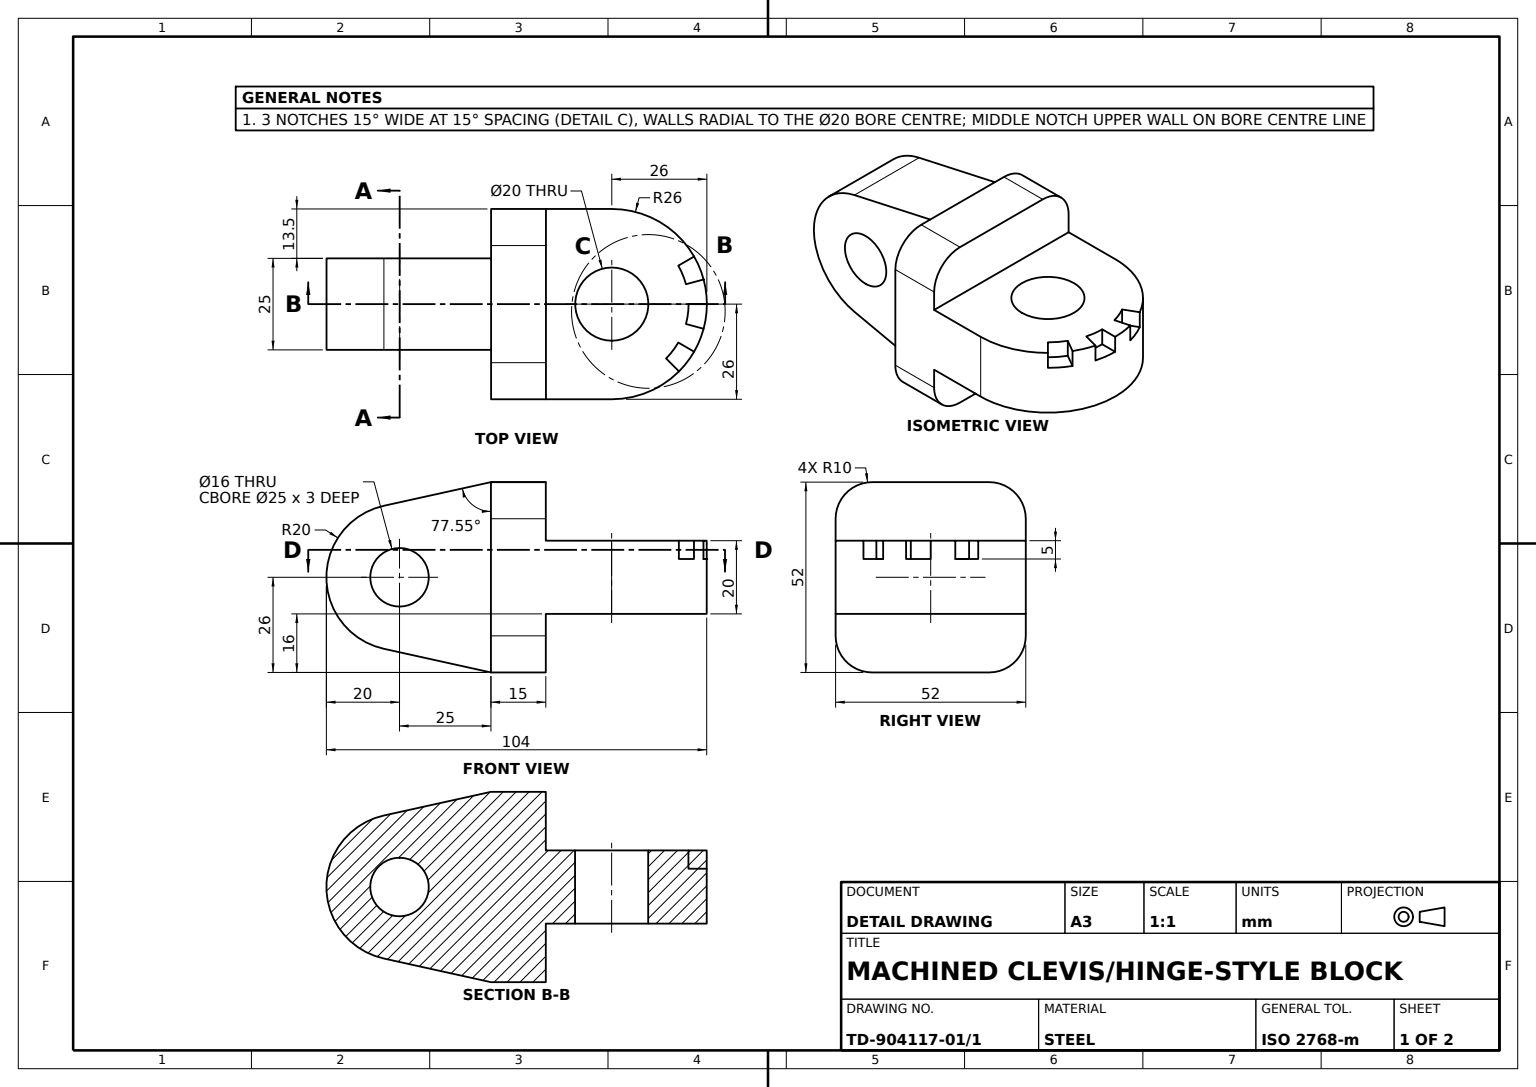
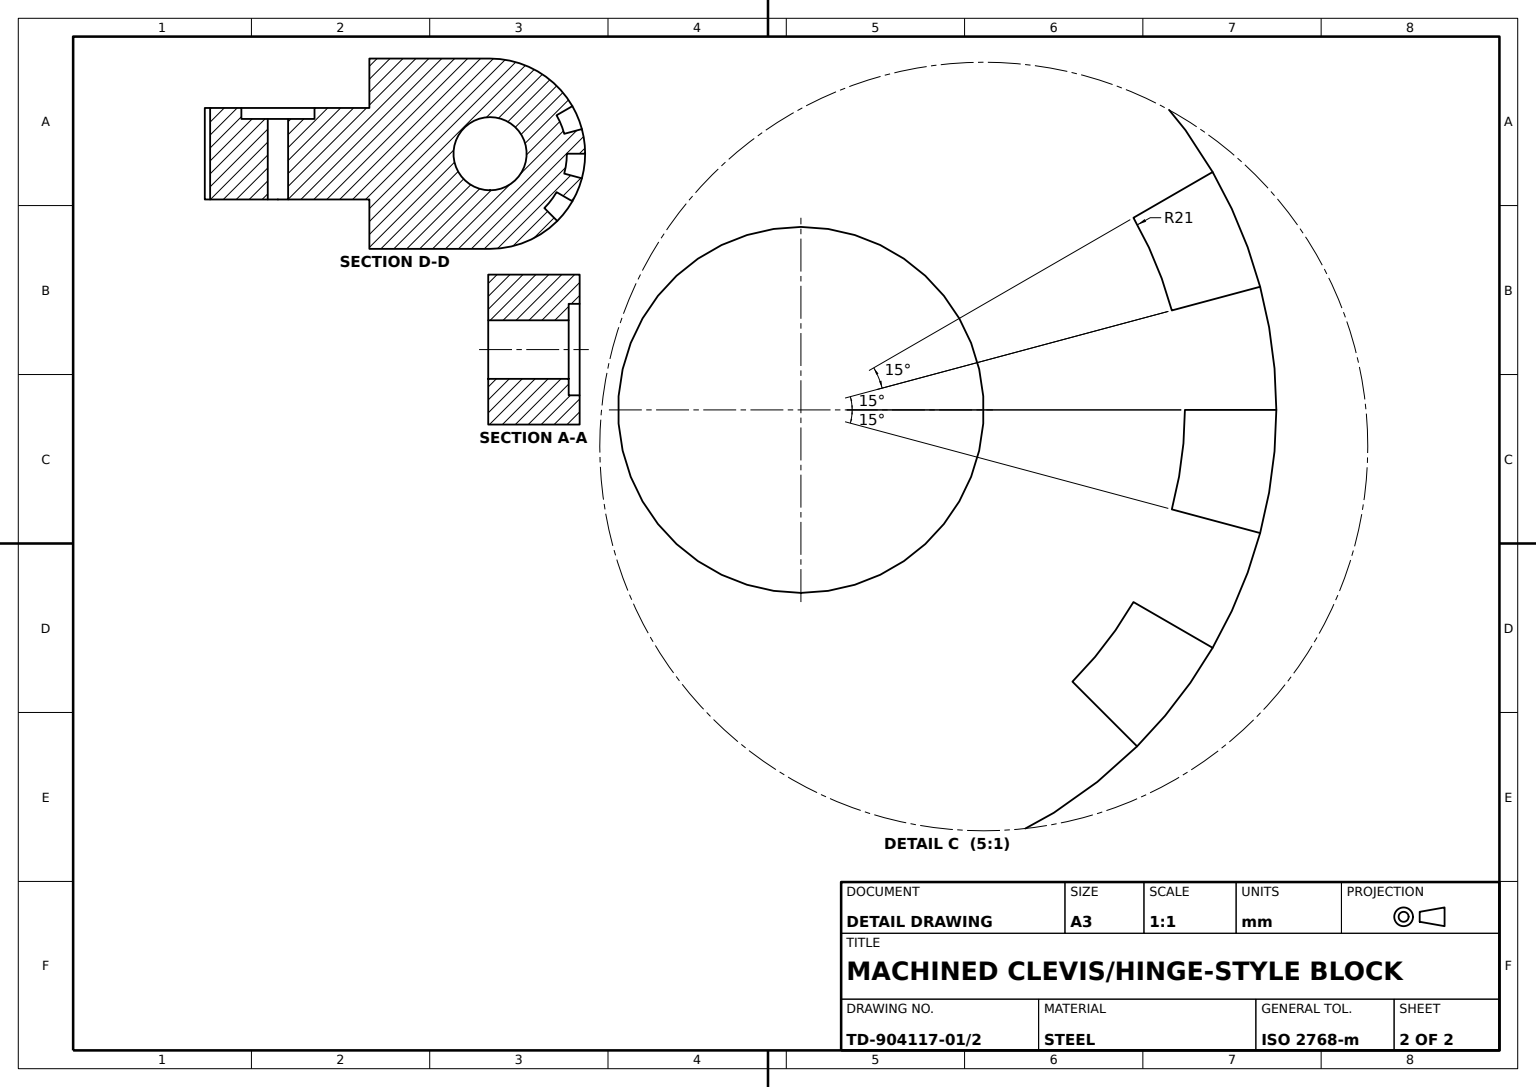
SolidWorks part; units mm, degrees
material "Plain Carbon Steel"
ref_plane "Front Plane" through (0, 0, 0) normal (0, 0, 1) x (1, 0, 0)
ref_plane "Top Plane" through (0, 0, 0) normal (0, 1, 0) x (1, 0, 0)
ref_plane "Right Plane" through (0, 0, 0) normal (1, 0, 0) x (0, 0, -1)
sketch "Base Block Profile Sketch" plane through (0, 0, 0) normal (0, 0, 1) x (1, 0, 0)
  line L0 (-16, 0) -> (16, 0)
  line L1 (26, 10) -> (26, 42)
  line L2 (16, 52) -> (-16, 52)
  line L3 (-26, 42) -> (-26, 10)
  arc A0 (-16, 0) -> (-26, 10) centre (-16, 10) cw
  arc A1 (16, 0) -> (26, 10) centre (16, 10) ccw
  arc A2 (26, 42) -> (16, 52) centre (16, 42) ccw
  arc A3 (-16, 52) -> (-26, 42) centre (-16, 42) ccw
  point P4 (0, 0)
  point P11 (26, 0)
  point P14 (26, 52)
  point P17 (-26, 52)
  dimension "D3" = 10
  dimension "D1" = 52
  dimension "D2" = 52
extrude "Rounded Base Block" add sketch "Base Block Profile Sketch" along normal blind 15
sketch "Upper Block Profile Sketch" plane through (-26, 0, 0) normal (-1, 0, 0) x (0, 0, 1)
  line L0 (15, 52) -> (15, 0)
  line L2 (15, 52) -> (44.311, 45.5298)
  line L3 (15, 0) -> (44.311, 6.4702)
  arc A0 (44.311, 6.4702) -> (44.311, 45.5298) centre (40, 26) ccw
  dimension "D2" = 20
  dimension "D1" = 25
  dimension "D3" = 19.5298
extrude "Upper Block" add sketch "Upper Block Profile Sketch" against normal blind 52
sketch "Upper Block Notch A Sketch" plane through (-26, 0, 0) normal (-1, 0, 0) x (0, 0, 1)
  line L0 (15, 52) -> (44.311, 45.5298)
  line L1 (15, 0) -> (44.311, 6.4702)
  line L2 (15, 52) -> (15, 0)
  arc A0 (44.311, 6.4702) -> (44.311, 45.5298) centre (40, 26) ccw
extrude "Upper Block Notch A" cut sketch "Upper Block Notch A Sketch" against normal blind 13.5
sketch "Upper Block Notch B Sketch" plane through (26, 0, 0) normal (1, 0, 0) x (0, 0, -1)
  line L0 (-15, 52) -> (-15, 0)
  line L1 (-15, 0) -> (-44.311, 6.4702)
  line L2 (-15, 52) -> (-44.311, 45.5298)
  arc A0 (-44.311, 45.5298) -> (-44.311, 6.4702) centre (-40, 26) ccw
extrude "Upper Block Notch B" cut sketch "Upper Block Notch B Sketch" against normal blind 13.5
sketch "Cross Block Profile Sketch" plane through (0, 52, 0) normal (0, 1, 0) x (1, 0, 0)
  line L1 (-26, 0) -> (-26, 18)
  line L2 (26, 0) -> (26, 18)
  line L3 (-26, 0) -> (26, 0)
  arc A0 (26, 18) -> (-26, 18) centre (0, 18) ccw
  dimension "D2" = 26
  dimension "D1" = 18
  dimension "D3" = 33
  dimension "D4" = 38.5
  dimension "D5" = 18
extrude "Cross Block" add sketch "Cross Block Profile Sketch" against normal blind 52
sketch "Cross Block Notch A Sketch" plane through (0, 52, 0) normal (0, 1, 0) x (1, 0, 0)
  line L0 (-26, 0) -> (26, 0)
  line L1 (26, 0) -> (26, 18)
  line L2 (-26, 0) -> (-26, 18)
  arc A0 (26, 18) -> (-26, 18) centre (0, 18) ccw
extrude "Cross Block Notch A" cut sketch "Cross Block Notch A Sketch" against normal blind 16
sketch "Cross Block Notch B Sketch" plane through (0, 0, 0) normal (0, -1, 0) x (1, 0, 0)
  line L0 (-26, 0) -> (26, 0)
  line L1 (26, 0) -> (26, -18)
  line L2 (-26, 0) -> (-26, -18)
  arc A0 (-26, -18) -> (26, -18) centre (0, -18) ccw
extrude "Cross Block Notch B" cut sketch "Cross Block Notch B Sketch" against normal blind 16
sketch "Bore Notch Teeth Sketch" plane through (0, 36, 0) normal (0, 1, 0) x (1, 0, 0)
  line L0 (0, 0) -> (0, 44)
  line L2 (-5.4352, 38.2844) -> (-6.7293, 43.1141)
  line L3 (5.4352, 38.2844) -> (6.7293, 43.1141)
  line L5 (-10.5, 36.1865) -> (-13, 40.5167)
  line L6 (14.8492, 32.8492) -> (18.3848, 36.3848)
  line L7 (10.5, 36.1865) -> (13, 40.5167)
  arc A0 (26, 18) -> (-26, 18) centre (0, 18) ccw construction
  arc A3 (14.8492, 32.8492) -> (10.5, 36.1865) centre (0, 18) ccw
  arc A4 (-5.4352, 38.2844) -> (-10.5, 36.1865) centre (0, 18) ccw
  arc A5 (18.3848, 36.3848) -> (13, 40.5167) centre (0, 18) ccw
  arc A6 (-6.7293, 43.1141) -> (-13, 40.5167) centre (0, 18) ccw
  arc A7 (5.4352, 38.2844) -> (0, 39) centre (0, 18) ccw
  arc A8 (6.7293, 43.1141) -> (0, 44) centre (0, 18) ccw
  arc M12 (26, 18) -> (-26, 18) centre (0, 18) ccw
  dimension "D1" = 15
  dimension "D3" = 15
  dimension "D7" = 21
  dimension "D2" = 15
  dimension "D4" = 15
  dimension "D5" = 75
  dimension "D6" = 4.3301
  dimension "D8" = 7.5648
  dimension "D9" = 13.0882
  dimension "D10" = 5
  dimension "D11" = 3.5355
extrude "Bore Notch Teeth Cut" cut sketch "Bore Notch Teeth Sketch" against normal blind 5 contours A4 L2 L5 M12 | A7 L3 L0 M12 | A3 L6 L7 M12
sketch "Cross Bore Ø10 Sketch" plane through (0, 36, 0) normal (0, 1, 0) x (1, 0, 0)
  circle A0 centre (0, 18) radius 10
  dimension "D1" = 10
extrude "Cross Bore Ø10" cut sketch "Cross Bore Ø10 Sketch" against normal blind 50
sketch "Counterbore Ø25 Sketch" plane through (-12.5, 0, 0) normal (-1, 0, 0) x (0, 0, 1)
  circle A0 centre (40, 26) radius 12.5
  dimension "D1" = 25
extrude "Counterbore Ø25 x3" cut sketch "Counterbore Ø25 Sketch" against normal blind 3
sketch "Main Bore Ø16 Sketch" plane through (-9.5, 0, 0) normal (-1, 0, 0) x (0, 0, 1)
  circle A0 centre (40, 26) radius 8
  dimension "D1" = 16
extrude "Main Bore Ø16" cut sketch "Main Bore Ø16 Sketch" against normal blind 50
